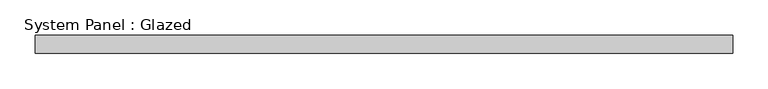
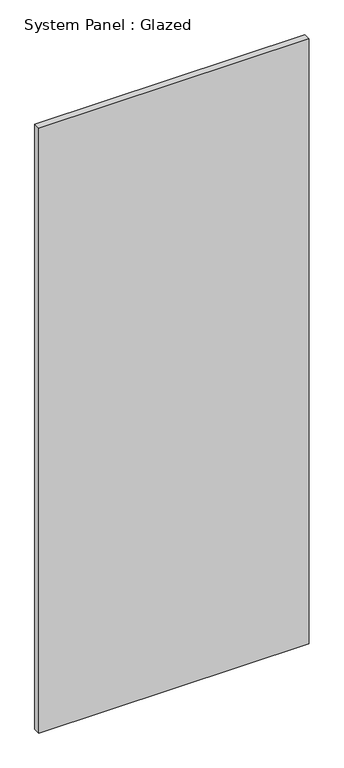
"""IFC4 building model written with IfcOpenShell, lengths in millimetres: plate geometry, System Panel : Glazed."""

from ifc_helpers import new_model, si_unit, origin, origin_with_axes, place, context, project, spatial, polyline, outline, extrude, source, transform, mapped, element, save


def system_panel_glazed_a992b757(model_context):
    return source(origin(), model_context, "Body", "SweptSolid", [
        extrude(outline(polyline([(495.3, 19.05), (-495.3, 19.05), (-495.3, 44.45), (495.3, 44.45), (495.3, 19.05)])), origin_with_axes(), (0.0, 0.0, 1.0), 2343.15),
    ])


if __name__ == "__main__":
    model = new_model("IFC4")
    model_context = context("Model", 3, world=origin())
    ifc_project = project(units=[si_unit("LENGTHUNIT", "METRE", prefix="MILLI")], contexts=[model_context])
    site = spatial("IfcSite", under=ifc_project)
    building = spatial("IfcBuilding", under=site)
    placement = place(None, origin())
    system_panel_glazed_shape = system_panel_glazed_a992b757(model_context)
    element("IfcPlate", 1, ObjectType="System Panel : Glazed", at=placement, inside=building, context=model_context, shape_type="MappedRepresentation", body=[
        mapped(system_panel_glazed_shape, transform((0.0, 0.0, 0.0), x_axis=(1.0, 0.0, 0.0), y_axis=(0.0, 1.0, 0.0), z_axis=(0.0, 0.0, 1.0))),
    ])
    save(model, "model.ifc")

# Revit data of these elements
# Type "System Panel : Glazed"
#   Construction Type Id = "GSP4R"
#   Analytic Construction = "1/8 in Pilkington single glazing"
#   Visual Light Transmittance = 0.9
#   Solar Heat Gain Coefficient = 0.86
#   Heat Transfer Coefficient (U) = 1.18115 BTU/(h·ft²·°F)
#   Define Thermal Properties by = 1
# Element 1 (IfcPlate, "System Panel : Glazed")
#   Materials on its faces: "Glass"
# Materials
#   "Glass": class "Glass", colour RGB 0 128 192, transparency 0.75, Description = "Soda Lime Glass", Cost = 0
